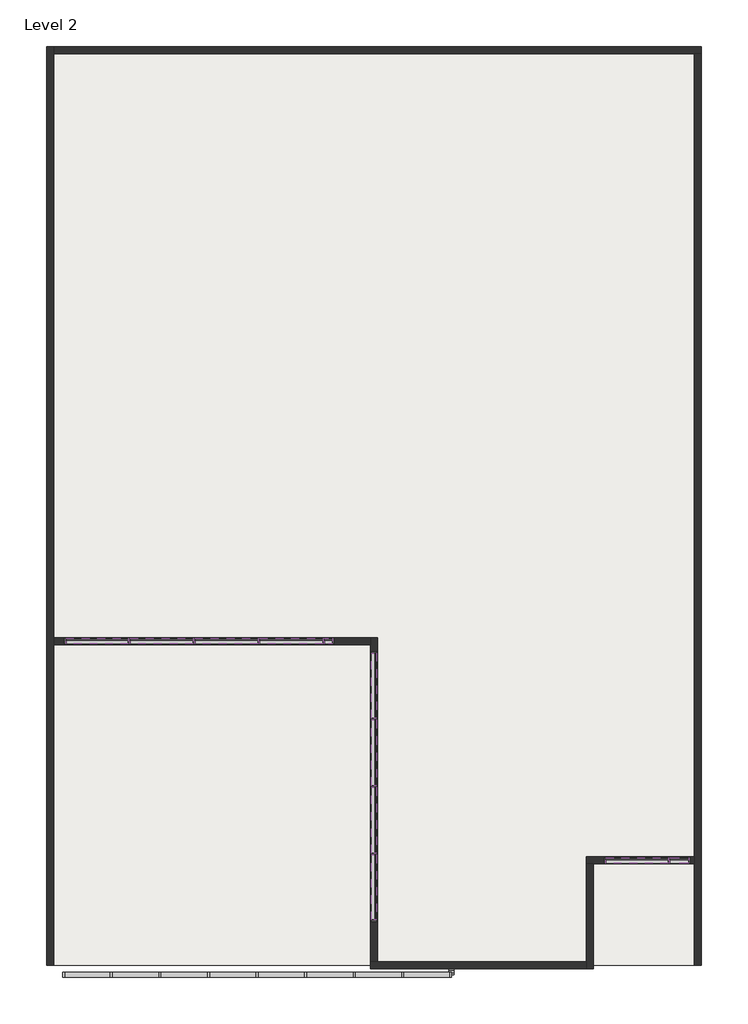
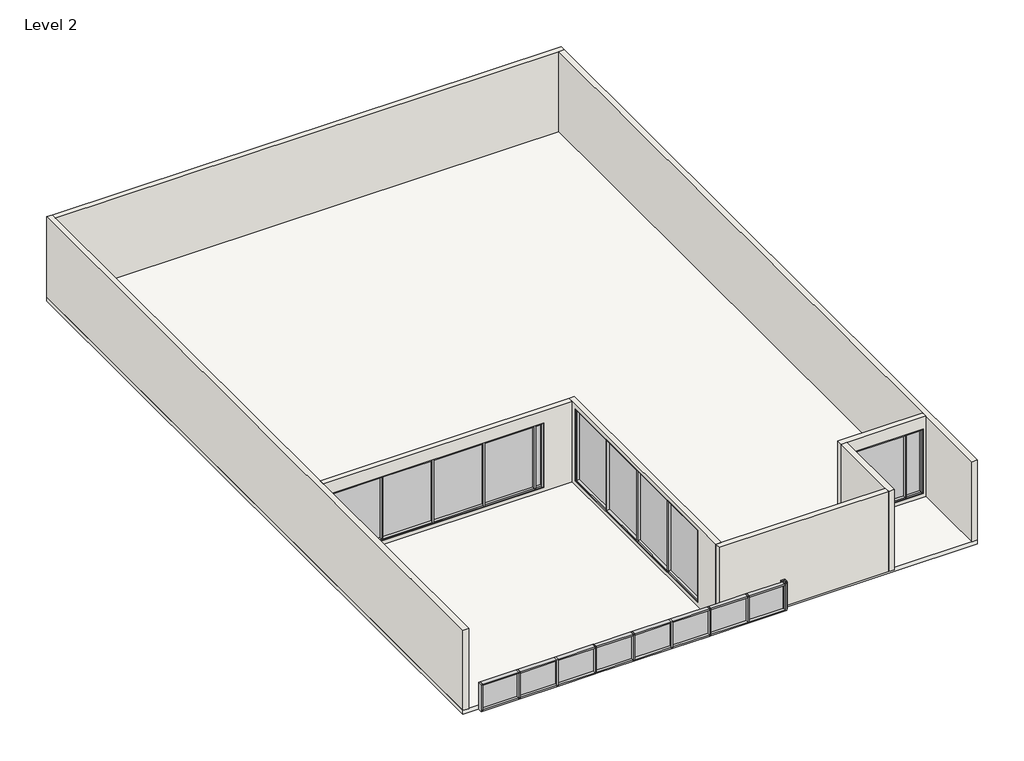
# One storey: 65 members, 20 plates, 8 walls, 1 slab.
"""IFC4 building model written with IfcOpenShell, lengths in millimetres."""

from ifc_helpers import new_model, si_unit, frame, origin, place, context, project, spatial, polyline, outline, extrude, faceted_brep, transform, mapped, element, save
from components import rectangular_mullion_50_x_150mm_ef1c4831, rectangular_mullion_50_x_150mm_86d49a4b, rectangular_mullion_50_x_150mm_a98d9a75, rectangular_mullion_50_x_150mm_ded00a16, rectangular_mullion_50_x_150mm_4a8db126, rectangular_mullion_50_x_150mm_15474f2d, rectangular_mullion_50_x_150mm_817551cd, rectangular_mullion_50_x_150mm_b402127a, rectangular_mullion_50_x_150mm_e4d4a7e6, rectangular_mullion_50_x_150mm_37458a5b, rectangular_mullion_50_x_150mm_e4b12c2e, rectangular_mullion_50_x_150mm_aaee7d48, rectangular_mullion_50_x_150mm_bcca0aad, rectangular_mullion_50_x_150mm_17218063, rectangular_mullion_50_x_150mm_0da89c4c, system_panel_glazed_91d575af, system_panel_glazed_99388aa9, system_panel_glazed_e22c965b, system_panel_glazed_90abe38c, system_panel_glazed_0f6e2381, system_panel_glazed_dc01897a, system_panel_glazed_f67349ae, system_panel_glazed_96f1d4d6, system_panel_glazed_c01e4bb7

model = new_model("IFC4")

# Units and contexts
model_context = context("Model", 3, world=origin())
ifc_project = project(units=[si_unit("LENGTHUNIT", "METRE", prefix="MILLI")], contexts=[model_context])

# Site, building, storey
site = spatial("IfcSite", under=ifc_project)
building = spatial("IfcBuilding", under=site)
storey = spatial("IfcBuildingStorey", under=building, Name="Level 2", Elevation=3048.0)

# Members
placement = place(None, origin())
rectangular_mullion_50_x_150mm_shape = rectangular_mullion_50_x_150mm_ef1c4831(model_context)
element("IfcMember", 1, ObjectType="Rectangular Mullion : 50 x 150mm", at=placement, inside=storey, context=model_context, shape_type="MappedRepresentation", body=[
    mapped(rectangular_mullion_50_x_150mm_shape, transform((-653.222521, -6711.5467593, 5638.8), x_axis=(0.0, 0.0, 1.0), y_axis=(0.0, -1.0, 0.0), z_axis=(1.0, 0.0, 0.0))),
])
rectangular_mullion_50_x_150mm_2_shape = rectangular_mullion_50_x_150mm_86d49a4b(model_context)
element("IfcMember", 2, ObjectType="Rectangular Mullion : 50 x 150mm", at=placement, inside=storey, context=model_context, shape_type="MappedRepresentation", body=[
    mapped(rectangular_mullion_50_x_150mm_2_shape, transform((-8173.222521, -6711.5467593, 3200.4), x_axis=(0.0, 0.0, -1.0), y_axis=(0.0, -1.0, 0.0), z_axis=(-1.0, 0.0, 0.0))),
])
element("IfcMember", 3, ObjectType="Rectangular Mullion : 50 x 150mm", at=placement, inside=storey, context=model_context, shape_type="MappedRepresentation", body=[
    mapped(rectangular_mullion_50_x_150mm_2_shape, transform((7066.777479, -12898.0177849, 3200.4), x_axis=(0.0, 0.0, -1.0), y_axis=(0.0, -1.0, 0.0), z_axis=(-1.0, 0.0, 0.0))),
])
rectangular_mullion_50_x_150mm_3_shape = rectangular_mullion_50_x_150mm_a98d9a75(model_context)
element("IfcMember", 4, ObjectType="Rectangular Mullion : 50 x 150mm", at=placement, inside=storey, context=model_context, shape_type="MappedRepresentation", body=[
    mapped(rectangular_mullion_50_x_150mm_3_shape, transform((-6393.222521, -6711.5467593, 3200.4), x_axis=(1.0, 0.0, 0.0), y_axis=(0.0, -1.0, 0.0), z_axis=(0.0, 0.0, -1.0))),
])
element("IfcMember", 5, ObjectType="Rectangular Mullion : 50 x 150mm", at=placement, inside=storey, context=model_context, shape_type="MappedRepresentation", body=[
    mapped(rectangular_mullion_50_x_150mm_3_shape, transform((-4563.222521, -6711.5467593, 3200.4), x_axis=(1.0, 0.0, 0.0), y_axis=(0.0, -1.0, 0.0), z_axis=(0.0, 0.0, -1.0))),
])
element("IfcMember", 6, ObjectType="Rectangular Mullion : 50 x 150mm", at=placement, inside=storey, context=model_context, shape_type="MappedRepresentation", body=[
    mapped(rectangular_mullion_50_x_150mm_3_shape, transform((-2733.222521, -6711.5467593, 3200.4), x_axis=(1.0, 0.0, 0.0), y_axis=(0.0, -1.0, 0.0), z_axis=(0.0, 0.0, -1.0))),
])
element("IfcMember", 7, ObjectType="Rectangular Mullion : 50 x 150mm", at=placement, inside=storey, context=model_context, shape_type="MappedRepresentation", body=[
    mapped(rectangular_mullion_50_x_150mm_3_shape, transform((-903.222521, -6711.5467593, 3200.4), x_axis=(1.0, 0.0, 0.0), y_axis=(0.0, -1.0, 0.0), z_axis=(0.0, 0.0, -1.0))),
])
element("IfcMember", 8, ObjectType="Rectangular Mullion : 50 x 150mm", at=placement, inside=storey, context=model_context, shape_type="MappedRepresentation", body=[
    mapped(rectangular_mullion_50_x_150mm_3_shape, transform((8846.777479, -12898.0177849, 3200.4), x_axis=(1.0, 0.0, 0.0), y_axis=(0.0, -1.0, 0.0), z_axis=(0.0, 0.0, -1.0))),
])
rectangular_mullion_50_x_150mm_4_shape = rectangular_mullion_50_x_150mm_ded00a16(model_context)
element("IfcMember", 9, ObjectType="Rectangular Mullion : 50 x 150mm", at=placement, inside=storey, context=model_context, shape_type="MappedRepresentation", body=[
    mapped(rectangular_mullion_50_x_150mm_4_shape, transform((-6368.222521, -6711.5467593, 3200.4), x_axis=(0.0, 0.0, -1.0), y_axis=(0.0, -1.0, 0.0), z_axis=(-1.0, 0.0, 0.0))),
])
element("IfcMember", 10, ObjectType="Rectangular Mullion : 50 x 150mm", at=placement, inside=storey, context=model_context, shape_type="MappedRepresentation", body=[
    mapped(rectangular_mullion_50_x_150mm_4_shape, transform((-4538.222521, -6711.5467593, 3200.4), x_axis=(0.0, 0.0, -1.0), y_axis=(0.0, -1.0, 0.0), z_axis=(-1.0, 0.0, 0.0))),
])
element("IfcMember", 11, ObjectType="Rectangular Mullion : 50 x 150mm", at=placement, inside=storey, context=model_context, shape_type="MappedRepresentation", body=[
    mapped(rectangular_mullion_50_x_150mm_4_shape, transform((-2708.222521, -6711.5467593, 3200.4), x_axis=(0.0, 0.0, -1.0), y_axis=(0.0, -1.0, 0.0), z_axis=(-1.0, 0.0, 0.0))),
])
element("IfcMember", 12, ObjectType="Rectangular Mullion : 50 x 150mm", at=placement, inside=storey, context=model_context, shape_type="MappedRepresentation", body=[
    mapped(rectangular_mullion_50_x_150mm_shape, transform((-878.222521, -6711.5467593, 3200.4), x_axis=(0.0, 0.0, -1.0), y_axis=(0.0, -1.0, 0.0), z_axis=(-1.0, 0.0, 0.0))),
])
element("IfcMember", 13, ObjectType="Rectangular Mullion : 50 x 150mm", at=placement, inside=storey, context=model_context, shape_type="MappedRepresentation", body=[
    mapped(rectangular_mullion_50_x_150mm_2_shape, transform((-6418.222521, -6711.5467593, 5638.8), x_axis=(0.0, 0.0, 1.0), y_axis=(0.0, -1.0, 0.0), z_axis=(1.0, 0.0, 0.0))),
])
element("IfcMember", 14, ObjectType="Rectangular Mullion : 50 x 150mm", at=placement, inside=storey, context=model_context, shape_type="MappedRepresentation", body=[
    mapped(rectangular_mullion_50_x_150mm_2_shape, transform((8821.777479, -12898.0177849, 5638.8), x_axis=(0.0, 0.0, 1.0), y_axis=(0.0, -1.0, 0.0), z_axis=(1.0, 0.0, 0.0))),
])
element("IfcMember", 15, ObjectType="Rectangular Mullion : 50 x 150mm", at=placement, inside=storey, context=model_context, shape_type="MappedRepresentation", body=[
    mapped(rectangular_mullion_50_x_150mm_4_shape, transform((-4588.222521, -6711.5467593, 5638.8), x_axis=(0.0, 0.0, 1.0), y_axis=(0.0, -1.0, 0.0), z_axis=(1.0, 0.0, 0.0))),
])
element("IfcMember", 16, ObjectType="Rectangular Mullion : 50 x 150mm", at=placement, inside=storey, context=model_context, shape_type="MappedRepresentation", body=[
    mapped(rectangular_mullion_50_x_150mm_4_shape, transform((-2758.222521, -6711.5467593, 5638.8), x_axis=(0.0, 0.0, 1.0), y_axis=(0.0, -1.0, 0.0), z_axis=(1.0, 0.0, 0.0))),
])
element("IfcMember", 17, ObjectType="Rectangular Mullion : 50 x 150mm", at=placement, inside=storey, context=model_context, shape_type="MappedRepresentation", body=[
    mapped(rectangular_mullion_50_x_150mm_4_shape, transform((-928.222521, -6711.5467593, 5638.8), x_axis=(0.0, 0.0, 1.0), y_axis=(0.0, -1.0, 0.0), z_axis=(1.0, 0.0, 0.0))),
])
rectangular_mullion_50_x_150mm_5_shape = rectangular_mullion_50_x_150mm_4a8db126(model_context)
element("IfcMember", 18, ObjectType="Rectangular Mullion : 50 x 150mm", at=placement, inside=storey, context=model_context, shape_type="MappedRepresentation", body=[
    mapped(rectangular_mullion_50_x_150mm_5_shape, transform((-8223.222521, -6711.5467593, 5638.8), x_axis=(-1.0, 0.0, 0.0), y_axis=(0.0, -1.0, 0.0), z_axis=(0.0, 0.0, 1.0))),
])
element("IfcMember", 19, ObjectType="Rectangular Mullion : 50 x 150mm", at=placement, inside=storey, context=model_context, shape_type="MappedRepresentation", body=[
    mapped(rectangular_mullion_50_x_150mm_5_shape, transform((7016.777479, -12898.0177849, 5638.8), x_axis=(-1.0, 0.0, 0.0), y_axis=(0.0, -1.0, 0.0), z_axis=(0.0, 0.0, 1.0))),
])
element("IfcMember", 20, ObjectType="Rectangular Mullion : 50 x 150mm", at=placement, inside=storey, context=model_context, shape_type="MappedRepresentation", body=[
    mapped(rectangular_mullion_50_x_150mm_5_shape, transform((-603.222521, -6711.5467593, 3200.4), x_axis=(1.0, 0.0, 0.0), y_axis=(0.0, -1.0, 0.0), z_axis=(0.0, 0.0, -1.0))),
])
element("IfcMember", 21, ObjectType="Rectangular Mullion : 50 x 150mm", at=placement, inside=storey, context=model_context, shape_type="MappedRepresentation", body=[
    mapped(rectangular_mullion_50_x_150mm_5_shape, transform((9455.177479, -12898.0177849, 3200.4), x_axis=(1.0, 0.0, 0.0), y_axis=(0.0, -1.0, 0.0), z_axis=(0.0, 0.0, -1.0))),
])
rectangular_mullion_50_x_150mm_6_shape = rectangular_mullion_50_x_150mm_15474f2d(model_context)
element("IfcMember", 22, ObjectType="Rectangular Mullion : 50 x 150mm", at=placement, inside=storey, context=model_context, shape_type="MappedRepresentation", body=[
    mapped(rectangular_mullion_50_x_150mm_6_shape, transform((9405.177479, -12898.0177849, 5638.8), x_axis=(0.0, 0.0, 1.0), y_axis=(0.0, -1.0, 0.0), z_axis=(1.0, 0.0, 0.0))),
])
element("IfcMember", 23, ObjectType="Rectangular Mullion : 50 x 150mm", at=placement, inside=storey, context=model_context, shape_type="MappedRepresentation", body=[
    mapped(rectangular_mullion_50_x_150mm_6_shape, transform((8871.777479, -12898.0177849, 3200.4), x_axis=(0.0, 0.0, -1.0), y_axis=(0.0, -1.0, 0.0), z_axis=(-1.0, 0.0, 0.0))),
])
rectangular_mullion_50_x_150mm_7_shape = rectangular_mullion_50_x_150mm_817551cd(model_context)
element("IfcMember", 24, ObjectType="Rectangular Mullion : 50 x 150mm", at=placement, inside=storey, context=model_context, shape_type="MappedRepresentation", body=[
    mapped(rectangular_mullion_50_x_150mm_7_shape, transform((2651.977479, -16123.9620478, 4075.5595785), x_axis=(0.0, 0.0, 1.0), y_axis=(0.0, -1.0, 0.0), z_axis=(1.0, 0.0, 0.0))),
])
element("IfcMember", 25, ObjectType="Rectangular Mullion : 50 x 150mm", at=placement, inside=storey, context=model_context, shape_type="MappedRepresentation", body=[
    mapped(rectangular_mullion_50_x_150mm_7_shape, transform((-6924.222521, -16123.9620478, 4075.5595785), x_axis=(0.0, 0.0, 1.0), y_axis=(0.0, -1.0, 0.0), z_axis=(1.0, 0.0, 0.0))),
])
element("IfcMember", 26, ObjectType="Rectangular Mullion : 50 x 150mm", at=placement, inside=storey, context=model_context, shape_type="MappedRepresentation", body=[
    mapped(rectangular_mullion_50_x_150mm_7_shape, transform((-8220.822521, -16123.9620478, 3048.0), x_axis=(0.0, 0.0, -1.0), y_axis=(0.0, -1.0, 0.0), z_axis=(-1.0, 0.0, 0.0))),
])
element("IfcMember", 27, ObjectType="Rectangular Mullion : 50 x 150mm", at=placement, inside=storey, context=model_context, shape_type="MappedRepresentation", body=[
    mapped(rectangular_mullion_50_x_150mm_7_shape, transform((1355.377479, -16123.9620478, 3048.0), x_axis=(0.0, 0.0, -1.0), y_axis=(0.0, -1.0, 0.0), z_axis=(-1.0, 0.0, 0.0))),
])
rectangular_mullion_50_x_150mm_8_shape = rectangular_mullion_50_x_150mm_b402127a(model_context)
element("IfcMember", 28, ObjectType="Rectangular Mullion : 50 x 150mm", at=placement, inside=storey, context=model_context, shape_type="MappedRepresentation", body=[
    mapped(rectangular_mullion_50_x_150mm_8_shape, transform((-2784.422521, -16123.9620478, 3048.0), x_axis=(1.0, 0.0, 0.0), y_axis=(0.0, -1.0, 0.0), z_axis=(0.0, 0.0, -1.0))),
])
element("IfcMember", 29, ObjectType="Rectangular Mullion : 50 x 150mm", at=placement, inside=storey, context=model_context, shape_type="MappedRepresentation", body=[
    mapped(rectangular_mullion_50_x_150mm_8_shape, transform((-5527.622521, -16123.9620478, 3048.0), x_axis=(1.0, 0.0, 0.0), y_axis=(0.0, -1.0, 0.0), z_axis=(0.0, 0.0, -1.0))),
])
element("IfcMember", 30, ObjectType="Rectangular Mullion : 50 x 150mm", at=placement, inside=storey, context=model_context, shape_type="MappedRepresentation", body=[
    mapped(rectangular_mullion_50_x_150mm_8_shape, transform((-4156.022521, -16123.9620478, 3048.0), x_axis=(1.0, 0.0, 0.0), y_axis=(0.0, -1.0, 0.0), z_axis=(0.0, 0.0, -1.0))),
])
element("IfcMember", 31, ObjectType="Rectangular Mullion : 50 x 150mm", at=placement, inside=storey, context=model_context, shape_type="MappedRepresentation", body=[
    mapped(rectangular_mullion_50_x_150mm_8_shape, transform((-6899.222521, -16123.9620478, 3048.0), x_axis=(1.0, 0.0, 0.0), y_axis=(0.0, -1.0, 0.0), z_axis=(0.0, 0.0, -1.0))),
])
element("IfcMember", 32, ObjectType="Rectangular Mullion : 50 x 150mm", at=placement, inside=storey, context=model_context, shape_type="MappedRepresentation", body=[
    mapped(rectangular_mullion_50_x_150mm_8_shape, transform((-1412.822521, -16123.9620478, 3048.0), x_axis=(1.0, 0.0, 0.0), y_axis=(0.0, -1.0, 0.0), z_axis=(0.0, 0.0, -1.0))),
])
element("IfcMember", 33, ObjectType="Rectangular Mullion : 50 x 150mm", at=placement, inside=storey, context=model_context, shape_type="MappedRepresentation", body=[
    mapped(rectangular_mullion_50_x_150mm_8_shape, transform((-41.222521, -16123.9620478, 3048.0), x_axis=(1.0, 0.0, 0.0), y_axis=(0.0, -1.0, 0.0), z_axis=(0.0, 0.0, -1.0))),
])
element("IfcMember", 34, ObjectType="Rectangular Mullion : 50 x 150mm", at=placement, inside=storey, context=model_context, shape_type="MappedRepresentation", body=[
    mapped(rectangular_mullion_50_x_150mm_8_shape, transform((1330.377479, -16123.9620478, 3048.0), x_axis=(1.0, 0.0, 0.0), y_axis=(0.0, -1.0, 0.0), z_axis=(0.0, 0.0, -1.0))),
])
rectangular_mullion_50_x_150mm_9_shape = rectangular_mullion_50_x_150mm_e4d4a7e6(model_context)
element("IfcMember", 35, ObjectType="Rectangular Mullion : 50 x 150mm", at=placement, inside=storey, context=model_context, shape_type="MappedRepresentation", body=[
    mapped(rectangular_mullion_50_x_150mm_9_shape, transform((-2759.422521, -16123.9620478, 3048.0), x_axis=(0.0, 0.0, -1.0), y_axis=(0.0, -1.0, 0.0), z_axis=(-1.0, 0.0, 0.0))),
])
element("IfcMember", 36, ObjectType="Rectangular Mullion : 50 x 150mm", at=placement, inside=storey, context=model_context, shape_type="MappedRepresentation", body=[
    mapped(rectangular_mullion_50_x_150mm_9_shape, transform((-5502.622521, -16123.9620478, 3048.0), x_axis=(0.0, 0.0, -1.0), y_axis=(0.0, -1.0, 0.0), z_axis=(-1.0, 0.0, 0.0))),
])
element("IfcMember", 37, ObjectType="Rectangular Mullion : 50 x 150mm", at=placement, inside=storey, context=model_context, shape_type="MappedRepresentation", body=[
    mapped(rectangular_mullion_50_x_150mm_9_shape, transform((-4131.022521, -16123.9620478, 3048.0), x_axis=(0.0, 0.0, -1.0), y_axis=(0.0, -1.0, 0.0), z_axis=(-1.0, 0.0, 0.0))),
])
element("IfcMember", 38, ObjectType="Rectangular Mullion : 50 x 150mm", at=placement, inside=storey, context=model_context, shape_type="MappedRepresentation", body=[
    mapped(rectangular_mullion_50_x_150mm_9_shape, transform((-6874.222521, -16123.9620478, 3048.0), x_axis=(0.0, 0.0, -1.0), y_axis=(0.0, -1.0, 0.0), z_axis=(-1.0, 0.0, 0.0))),
])
element("IfcMember", 39, ObjectType="Rectangular Mullion : 50 x 150mm", at=placement, inside=storey, context=model_context, shape_type="MappedRepresentation", body=[
    mapped(rectangular_mullion_50_x_150mm_9_shape, transform((-1387.822521, -16123.9620478, 3048.0), x_axis=(0.0, 0.0, -1.0), y_axis=(0.0, -1.0, 0.0), z_axis=(-1.0, 0.0, 0.0))),
])
element("IfcMember", 40, ObjectType="Rectangular Mullion : 50 x 150mm", at=placement, inside=storey, context=model_context, shape_type="MappedRepresentation", body=[
    mapped(rectangular_mullion_50_x_150mm_9_shape, transform((-16.222521, -16123.9620478, 3048.0), x_axis=(0.0, 0.0, -1.0), y_axis=(0.0, -1.0, 0.0), z_axis=(-1.0, 0.0, 0.0))),
])
element("IfcMember", 41, ObjectType="Rectangular Mullion : 50 x 150mm", at=placement, inside=storey, context=model_context, shape_type="MappedRepresentation", body=[
    mapped(rectangular_mullion_50_x_150mm_9_shape, transform((-2809.422521, -16123.9620478, 4075.5595785), x_axis=(0.0, 0.0, 1.0), y_axis=(0.0, -1.0, 0.0), z_axis=(1.0, 0.0, 0.0))),
])
element("IfcMember", 42, ObjectType="Rectangular Mullion : 50 x 150mm", at=placement, inside=storey, context=model_context, shape_type="MappedRepresentation", body=[
    mapped(rectangular_mullion_50_x_150mm_9_shape, transform((-5552.622521, -16123.9620478, 4075.5595785), x_axis=(0.0, 0.0, 1.0), y_axis=(0.0, -1.0, 0.0), z_axis=(1.0, 0.0, 0.0))),
])
element("IfcMember", 43, ObjectType="Rectangular Mullion : 50 x 150mm", at=placement, inside=storey, context=model_context, shape_type="MappedRepresentation", body=[
    mapped(rectangular_mullion_50_x_150mm_9_shape, transform((-4181.022521, -16123.9620478, 4075.5595785), x_axis=(0.0, 0.0, 1.0), y_axis=(0.0, -1.0, 0.0), z_axis=(1.0, 0.0, 0.0))),
])
element("IfcMember", 44, ObjectType="Rectangular Mullion : 50 x 150mm", at=placement, inside=storey, context=model_context, shape_type="MappedRepresentation", body=[
    mapped(rectangular_mullion_50_x_150mm_9_shape, transform((-1437.822521, -16123.9620478, 4075.5595785), x_axis=(0.0, 0.0, 1.0), y_axis=(0.0, -1.0, 0.0), z_axis=(1.0, 0.0, 0.0))),
])
element("IfcMember", 45, ObjectType="Rectangular Mullion : 50 x 150mm", at=placement, inside=storey, context=model_context, shape_type="MappedRepresentation", body=[
    mapped(rectangular_mullion_50_x_150mm_9_shape, transform((-66.222521, -16123.9620478, 4075.5595785), x_axis=(0.0, 0.0, 1.0), y_axis=(0.0, -1.0, 0.0), z_axis=(1.0, 0.0, 0.0))),
])
element("IfcMember", 46, ObjectType="Rectangular Mullion : 50 x 150mm", at=placement, inside=storey, context=model_context, shape_type="MappedRepresentation", body=[
    mapped(rectangular_mullion_50_x_150mm_9_shape, transform((1305.377479, -16123.9620478, 4075.5595785), x_axis=(0.0, 0.0, 1.0), y_axis=(0.0, -1.0, 0.0), z_axis=(1.0, 0.0, 0.0))),
])
rectangular_mullion_50_x_150mm_10_shape = rectangular_mullion_50_x_150mm_37458a5b(model_context)
element("IfcMember", 47, ObjectType="Rectangular Mullion : 50 x 150mm", at=placement, inside=storey, context=model_context, shape_type="MappedRepresentation", body=[
    mapped(rectangular_mullion_50_x_150mm_10_shape, transform((-8270.822521, -16123.9620478, 4075.5595785), x_axis=(-1.0, 0.0, 0.0), y_axis=(0.0, -1.0, 0.0), z_axis=(0.0, 0.0, 1.0))),
])
element("IfcMember", 48, ObjectType="Rectangular Mullion : 50 x 150mm", at=placement, inside=storey, context=model_context, shape_type="MappedRepresentation", body=[
    mapped(rectangular_mullion_50_x_150mm_10_shape, transform((2701.977479, -16123.9620478, 4075.5595785), x_axis=(0.0, -1.0, 0.0), y_axis=(1.0, 0.0, 0.0), z_axis=(0.0, 0.0, 1.0))),
])
element("IfcMember", 49, ObjectType="Rectangular Mullion : 50 x 150mm", at=placement, inside=storey, context=model_context, shape_type="MappedRepresentation", body=[
    mapped(rectangular_mullion_50_x_150mm_10_shape, transform((2701.977479, -16123.9620478, 3048.0), x_axis=(1.0, 0.0, 0.0), y_axis=(0.0, -1.0, 0.0), z_axis=(0.0, 0.0, -1.0))),
])
element("IfcMember", 50, ObjectType="Rectangular Mullion : 50 x 150mm", at=placement, inside=storey, context=model_context, shape_type="MappedRepresentation", body=[
    mapped(rectangular_mullion_50_x_150mm_10_shape, transform((2701.977479, -15955.5467593, 3048.0), x_axis=(0.0, 1.0, 0.0), y_axis=(1.0, 0.0, 0.0), z_axis=(0.0, 0.0, -1.0))),
])
rectangular_mullion_50_x_150mm_11_shape = rectangular_mullion_50_x_150mm_e4b12c2e(model_context)
element("IfcMember", 51, ObjectType="Rectangular Mullion : 50 x 150mm", at=placement, inside=storey, context=model_context, shape_type="MappedRepresentation", body=[
    mapped(rectangular_mullion_50_x_150mm_11_shape, transform((2701.977479, -16005.5467593, 4075.5595785), x_axis=(0.0, 0.0, 1.0), y_axis=(1.0, 0.0, 0.0), z_axis=(0.0, 1.0, 0.0))),
])
element("IfcMember", 52, ObjectType="Rectangular Mullion : 50 x 150mm", at=placement, inside=storey, context=model_context, shape_type="MappedRepresentation", body=[
    mapped(rectangular_mullion_50_x_150mm_11_shape, transform((2701.977479, -16073.9620478, 3048.0), x_axis=(0.0, 0.0, -1.0), y_axis=(1.0, 0.0, 0.0), z_axis=(0.0, -1.0, 0.0))),
])
rectangular_mullion_50_x_150mm_12_shape = rectangular_mullion_50_x_150mm_aaee7d48(model_context)
element("IfcMember", 53, ObjectType="Rectangular Mullion : 50 x 150mm", at=placement, inside=storey, context=model_context, shape_type="MappedRepresentation", body=[
    mapped(rectangular_mullion_50_x_150mm_12_shape, transform((515.977479, -14573.2177849, 5943.6), x_axis=(0.0, 0.0, 1.0), y_axis=(-1.0, 0.0, 0.0), z_axis=(0.0, -1.0, 0.0))),
])
element("IfcMember", 54, ObjectType="Rectangular Mullion : 50 x 150mm", at=placement, inside=storey, context=model_context, shape_type="MappedRepresentation", body=[
    mapped(rectangular_mullion_50_x_150mm_12_shape, transform((515.977479, -8883.2177849, 5943.6), x_axis=(0.0, 0.0, 1.0), y_axis=(-1.0, 0.0, 0.0), z_axis=(0.0, -1.0, 0.0))),
])
element("IfcMember", 55, ObjectType="Rectangular Mullion : 50 x 150mm", at=placement, inside=storey, context=model_context, shape_type="MappedRepresentation", body=[
    mapped(rectangular_mullion_50_x_150mm_12_shape, transform((515.977479, -7053.2177849, 3200.4), x_axis=(0.0, 0.0, -1.0), y_axis=(-1.0, 0.0, 0.0), z_axis=(0.0, 1.0, 0.0))),
])
element("IfcMember", 56, ObjectType="Rectangular Mullion : 50 x 150mm", at=placement, inside=storey, context=model_context, shape_type="MappedRepresentation", body=[
    mapped(rectangular_mullion_50_x_150mm_12_shape, transform((515.977479, -12743.2177849, 3200.4), x_axis=(0.0, 0.0, -1.0), y_axis=(-1.0, 0.0, 0.0), z_axis=(0.0, 1.0, 0.0))),
])
rectangular_mullion_50_x_150mm_13_shape = rectangular_mullion_50_x_150mm_bcca0aad(model_context)
element("IfcMember", 57, ObjectType="Rectangular Mullion : 50 x 150mm", at=placement, inside=storey, context=model_context, shape_type="MappedRepresentation", body=[
    mapped(rectangular_mullion_50_x_150mm_13_shape, transform((515.977479, -10813.2177849, 3200.4), x_axis=(0.0, -1.0, 0.0), y_axis=(-1.0, 0.0, 0.0), z_axis=(0.0, 0.0, -1.0))),
])
element("IfcMember", 58, ObjectType="Rectangular Mullion : 50 x 150mm", at=placement, inside=storey, context=model_context, shape_type="MappedRepresentation", body=[
    mapped(rectangular_mullion_50_x_150mm_13_shape, transform((515.977479, -8908.2177849, 3200.4), x_axis=(0.0, -1.0, 0.0), y_axis=(-1.0, 0.0, 0.0), z_axis=(0.0, 0.0, -1.0))),
])
element("IfcMember", 59, ObjectType="Rectangular Mullion : 50 x 150mm", at=placement, inside=storey, context=model_context, shape_type="MappedRepresentation", body=[
    mapped(rectangular_mullion_50_x_150mm_13_shape, transform((515.977479, -12718.2177849, 3200.4), x_axis=(0.0, -1.0, 0.0), y_axis=(-1.0, 0.0, 0.0), z_axis=(0.0, 0.0, -1.0))),
])
rectangular_mullion_50_x_150mm_14_shape = rectangular_mullion_50_x_150mm_17218063(model_context)
element("IfcMember", 60, ObjectType="Rectangular Mullion : 50 x 150mm", at=placement, inside=storey, context=model_context, shape_type="MappedRepresentation", body=[
    mapped(rectangular_mullion_50_x_150mm_14_shape, transform((515.977479, -10838.2177849, 3200.4), x_axis=(0.0, 0.0, -1.0), y_axis=(-1.0, 0.0, 0.0), z_axis=(0.0, 1.0, 0.0))),
])
element("IfcMember", 61, ObjectType="Rectangular Mullion : 50 x 150mm", at=placement, inside=storey, context=model_context, shape_type="MappedRepresentation", body=[
    mapped(rectangular_mullion_50_x_150mm_14_shape, transform((515.977479, -8933.2177849, 3200.4), x_axis=(0.0, 0.0, -1.0), y_axis=(-1.0, 0.0, 0.0), z_axis=(0.0, 1.0, 0.0))),
])
element("IfcMember", 62, ObjectType="Rectangular Mullion : 50 x 150mm", at=placement, inside=storey, context=model_context, shape_type="MappedRepresentation", body=[
    mapped(rectangular_mullion_50_x_150mm_14_shape, transform((515.977479, -10788.2177849, 5943.6), x_axis=(0.0, 0.0, 1.0), y_axis=(-1.0, 0.0, 0.0), z_axis=(0.0, -1.0, 0.0))),
])
element("IfcMember", 63, ObjectType="Rectangular Mullion : 50 x 150mm", at=placement, inside=storey, context=model_context, shape_type="MappedRepresentation", body=[
    mapped(rectangular_mullion_50_x_150mm_14_shape, transform((515.977479, -12693.2177849, 5943.6), x_axis=(0.0, 0.0, 1.0), y_axis=(-1.0, 0.0, 0.0), z_axis=(0.0, -1.0, 0.0))),
])
rectangular_mullion_50_x_150mm_15_shape = rectangular_mullion_50_x_150mm_0da89c4c(model_context)
element("IfcMember", 64, ObjectType="Rectangular Mullion : 50 x 150mm", at=placement, inside=storey, context=model_context, shape_type="MappedRepresentation", body=[
    mapped(rectangular_mullion_50_x_150mm_15_shape, transform((515.977479, -7003.2177849, 5943.6), x_axis=(0.0, 1.0, 0.0), y_axis=(-1.0, 0.0, 0.0), z_axis=(0.0, 0.0, 1.0))),
])
element("IfcMember", 65, ObjectType="Rectangular Mullion : 50 x 150mm", at=placement, inside=storey, context=model_context, shape_type="MappedRepresentation", body=[
    mapped(rectangular_mullion_50_x_150mm_15_shape, transform((515.977479, -14623.2177849, 3200.4), x_axis=(0.0, -1.0, 0.0), y_axis=(-1.0, 0.0, 0.0), z_axis=(0.0, 0.0, -1.0))),
])

# Plates
system_panel_glazed_shape = system_panel_glazed_91d575af(model_context)
element("IfcPlate", 66, ObjectType="System Panel : Glazed", at=placement, inside=storey, context=model_context, shape_type="MappedRepresentation", body=[
    mapped(system_panel_glazed_shape, transform((-7295.722521, -6711.5467593, 3250.4), x_axis=(1.0, 0.0, 0.0), y_axis=(0.0, 1.0, 0.0), z_axis=(0.0, 0.0, 1.0))),
])
element("IfcPlate", 67, ObjectType="System Panel : Glazed", at=placement, inside=storey, context=model_context, shape_type="MappedRepresentation", body=[
    mapped(system_panel_glazed_shape, transform((7944.277479, -12898.0177849, 3250.4), x_axis=(1.0, 0.0, 0.0), y_axis=(0.0, 1.0, 0.0), z_axis=(0.0, 0.0, 1.0))),
])
system_panel_glazed_2_shape = system_panel_glazed_99388aa9(model_context)
element("IfcPlate", 68, ObjectType="System Panel : Glazed", at=placement, inside=storey, context=model_context, shape_type="MappedRepresentation", body=[
    mapped(system_panel_glazed_2_shape, transform((-5478.222521, -6711.5467593, 3250.4), x_axis=(1.0, 0.0, 0.0), y_axis=(0.0, 1.0, 0.0), z_axis=(0.0, 0.0, 1.0))),
])
element("IfcPlate", 69, ObjectType="System Panel : Glazed", at=placement, inside=storey, context=model_context, shape_type="MappedRepresentation", body=[
    mapped(system_panel_glazed_2_shape, transform((-3648.222521, -6711.5467593, 3250.4), x_axis=(1.0, 0.0, 0.0), y_axis=(0.0, 1.0, 0.0), z_axis=(0.0, 0.0, 1.0))),
])
element("IfcPlate", 70, ObjectType="System Panel : Glazed", at=placement, inside=storey, context=model_context, shape_type="MappedRepresentation", body=[
    mapped(system_panel_glazed_2_shape, transform((-1818.222521, -6711.5467593, 3250.4), x_axis=(1.0, 0.0, 0.0), y_axis=(0.0, 1.0, 0.0), z_axis=(0.0, 0.0, 1.0))),
])
system_panel_glazed_3_shape = system_panel_glazed_e22c965b(model_context)
element("IfcPlate", 71, ObjectType="System Panel : Glazed", at=placement, inside=storey, context=model_context, shape_type="MappedRepresentation", body=[
    mapped(system_panel_glazed_3_shape, transform((-765.722521, -6711.5467593, 3250.4), x_axis=(1.0, 0.0, 0.0), y_axis=(0.0, 1.0, 0.0), z_axis=(0.0, 0.0, 1.0))),
])
system_panel_glazed_4_shape = system_panel_glazed_90abe38c(model_context)
element("IfcPlate", 72, ObjectType="System Panel : Glazed", at=placement, inside=storey, context=model_context, shape_type="MappedRepresentation", body=[
    mapped(system_panel_glazed_4_shape, transform((9138.477479, -12898.0177849, 3250.4), x_axis=(1.0, 0.0, 0.0), y_axis=(0.0, 1.0, 0.0), z_axis=(0.0, 0.0, 1.0))),
])
system_panel_glazed_5_shape = system_panel_glazed_0f6e2381(model_context)
element("IfcPlate", 73, ObjectType="System Panel : Glazed", at=placement, inside=storey, context=model_context, shape_type="MappedRepresentation", body=[
    mapped(system_panel_glazed_5_shape, transform((-7572.522521, -16123.9620478, 3098.0), x_axis=(1.0, 0.0, 0.0), y_axis=(0.0, 1.0, 0.0), z_axis=(0.0, 0.0, 1.0))),
])
element("IfcPlate", 74, ObjectType="System Panel : Glazed", at=placement, inside=storey, context=model_context, shape_type="MappedRepresentation", body=[
    mapped(system_panel_glazed_5_shape, transform((2003.677479, -16123.9620478, 3098.0), x_axis=(1.0, 0.0, 0.0), y_axis=(0.0, 1.0, 0.0), z_axis=(0.0, 0.0, 1.0))),
])
system_panel_glazed_6_shape = system_panel_glazed_dc01897a(model_context)
element("IfcPlate", 75, ObjectType="System Panel : Glazed", at=placement, inside=storey, context=model_context, shape_type="MappedRepresentation", body=[
    mapped(system_panel_glazed_6_shape, transform((-2098.622521, -16123.9620478, 3098.0), x_axis=(1.0, 0.0, 0.0), y_axis=(0.0, 1.0, 0.0), z_axis=(0.0, 0.0, 1.0))),
])
element("IfcPlate", 76, ObjectType="System Panel : Glazed", at=placement, inside=storey, context=model_context, shape_type="MappedRepresentation", body=[
    mapped(system_panel_glazed_6_shape, transform((-4841.822521, -16123.9620478, 3098.0), x_axis=(1.0, 0.0, 0.0), y_axis=(0.0, 1.0, 0.0), z_axis=(0.0, 0.0, 1.0))),
])
element("IfcPlate", 77, ObjectType="System Panel : Glazed", at=placement, inside=storey, context=model_context, shape_type="MappedRepresentation", body=[
    mapped(system_panel_glazed_6_shape, transform((-3470.222521, -16123.9620478, 3098.0), x_axis=(1.0, 0.0, 0.0), y_axis=(0.0, 1.0, 0.0), z_axis=(0.0, 0.0, 1.0))),
])
element("IfcPlate", 78, ObjectType="System Panel : Glazed", at=placement, inside=storey, context=model_context, shape_type="MappedRepresentation", body=[
    mapped(system_panel_glazed_6_shape, transform((-6213.422521, -16123.9620478, 3098.0), x_axis=(1.0, 0.0, 0.0), y_axis=(0.0, 1.0, 0.0), z_axis=(0.0, 0.0, 1.0))),
])
element("IfcPlate", 79, ObjectType="System Panel : Glazed", at=placement, inside=storey, context=model_context, shape_type="MappedRepresentation", body=[
    mapped(system_panel_glazed_6_shape, transform((-727.022521, -16123.9620478, 3098.0), x_axis=(1.0, 0.0, 0.0), y_axis=(0.0, 1.0, 0.0), z_axis=(0.0, 0.0, 1.0))),
])
element("IfcPlate", 80, ObjectType="System Panel : Glazed", at=placement, inside=storey, context=model_context, shape_type="MappedRepresentation", body=[
    mapped(system_panel_glazed_6_shape, transform((644.577479, -16123.9620478, 3098.0), x_axis=(1.0, 0.0, 0.0), y_axis=(0.0, 1.0, 0.0), z_axis=(0.0, 0.0, 1.0))),
])
system_panel_glazed_7_shape = system_panel_glazed_f67349ae(model_context)
element("IfcPlate", 81, ObjectType="System Panel : Glazed", at=placement, inside=storey, context=model_context, shape_type="MappedRepresentation", body=[
    mapped(system_panel_glazed_7_shape, transform((2701.977479, -16039.7544035, 3098.0), x_axis=(0.0, 1.0, 0.0), y_axis=(-1.0, 0.0, 0.0), z_axis=(0.0, 0.0, 1.0))),
])
system_panel_glazed_8_shape = system_panel_glazed_96f1d4d6(model_context)
element("IfcPlate", 82, ObjectType="System Panel : Glazed", at=placement, inside=storey, context=model_context, shape_type="MappedRepresentation", body=[
    mapped(system_panel_glazed_8_shape, transform((515.977479, -7968.2177849, 3250.4), x_axis=(0.0, -1.0, 0.0), y_axis=(1.0, 0.0, 0.0), z_axis=(0.0, 0.0, 1.0))),
])
element("IfcPlate", 83, ObjectType="System Panel : Glazed", at=placement, inside=storey, context=model_context, shape_type="MappedRepresentation", body=[
    mapped(system_panel_glazed_8_shape, transform((515.977479, -13658.2177849, 3250.4), x_axis=(0.0, -1.0, 0.0), y_axis=(1.0, 0.0, 0.0), z_axis=(0.0, 0.0, 1.0))),
])
system_panel_glazed_9_shape = system_panel_glazed_c01e4bb7(model_context)
element("IfcPlate", 84, ObjectType="System Panel : Glazed", at=placement, inside=storey, context=model_context, shape_type="MappedRepresentation", body=[
    mapped(system_panel_glazed_9_shape, transform((515.977479, -11765.7177849, 3250.4), x_axis=(0.0, -1.0, 0.0), y_axis=(1.0, 0.0, 0.0), z_axis=(0.0, 0.0, 1.0))),
])
element("IfcPlate", 85, ObjectType="System Panel : Glazed", at=placement, inside=storey, context=model_context, shape_type="MappedRepresentation", body=[
    mapped(system_panel_glazed_9_shape, transform((515.977479, -9860.7177849, 3250.4), x_axis=(0.0, -1.0, 0.0), y_axis=(1.0, 0.0, 0.0), z_axis=(0.0, 0.0, 1.0))),
])

# Slab
element("IfcSlab", 86, ObjectType="Generic 150mm", at=placement, inside=storey, context=model_context, shape_type="SweptSolid", body=[
    extrude(outline(polyline([(-8728.022521, 10061.9822151), (9759.977479, 10061.9822151), (9759.977479, -15855.5467593), (-8728.022521, -15855.5467593), (-8728.022521, 10061.9822151)])), frame((0.0, 0.0, 2895.6), z_axis=(0.0, 0.0, 1.0), x_axis=(1.0, 0.0, 0.0)), (0.0, 0.0, 1.0), 152.4),
])

# Walls
element("IfcWall", 87, ObjectType="Generic - 200mm", at=placement, inside=storey, context=model_context, shape_type="Brep", body=[
    faceted_brep([(-8728.022521, 10061.9822151, 3048.0), (-8728.022521, -15855.5467593, 3048.0), (-8728.022521, -15855.5467593, 6096.0), (-8728.022521, 10061.9822151, 6096.0), (-8528.022521, 10061.9822151, 3048.0), (-8528.022521, 10061.9822151, 6096.0), (-8528.022521, 9861.9822151, 6096.0), (-8528.022521, -6611.5467593, 6096.0), (-8528.022521, -6811.5467593, 6096.0), (-8528.022521, -15855.5467593, 6096.0), (-8528.022521, -15855.5467593, 3048.0), (-8528.022521, -6811.5467593, 3048.0), (-8528.022521, -6611.5467593, 3048.0), (-8528.022521, 9861.9822151, 3048.0)], [[[0, 1, 2, 3]], [[4, 5, 6, 7, 8, 9, 10, 11, 12, 13]], [[1, 0, 4, 13, 12, 11, 10]], [[2, 1, 10, 9]], [[3, 2, 9, 8, 7, 6, 5]], [[0, 3, 5, 4]]]),
])
element("IfcWall", 88, ObjectType="Generic - 200mm", at=placement, inside=storey, context=model_context, shape_type="Brep", body=[
    faceted_brep([(-8528.022521, 9861.9822151, 3048.0), (9559.977479, 9861.9822151, 3048.0), (9759.977479, 9861.9822151, 3048.0), (9759.977479, 9861.9822151, 6096.0), (9559.977479, 9861.9822151, 6096.0), (-8528.022521, 9861.9822151, 6096.0), (-8528.022521, 10061.9822151, 3048.0), (-8528.022521, 10061.9822151, 6096.0), (9759.977479, 10061.9822151, 6096.0), (9759.977479, 10061.9822151, 3048.0)], [[[0, 1, 2, 3, 4, 5]], [[6, 7, 8, 9]], [[2, 1, 0, 6, 9]], [[5, 4, 3, 8, 7]], [[0, 5, 7, 6]], [[3, 2, 9, 8]]]),
])
element("IfcWall", 89, ObjectType="Generic - 200mm", at=placement, inside=storey, context=model_context, shape_type="Brep", body=[
    faceted_brep([(9559.977479, 9861.9822151, 3048.0), (9559.977479, -12798.0177849, 3048.0), (9559.977479, -12998.0177849, 3048.0), (9559.977479, -15855.5467593, 3048.0), (9559.977479, -15855.5467593, 6096.0), (9559.977479, -12998.0177849, 6096.0), (9559.977479, -12798.0177849, 6096.0), (9559.977479, 9861.9822151, 6096.0), (9759.977479, 9861.9822151, 3048.0), (9759.977479, 9861.9822151, 6096.0), (9759.977479, -15855.5467593, 6096.0), (9759.977479, -15855.5467593, 3048.0)], [[[0, 1, 2, 3, 4, 5, 6, 7]], [[8, 9, 10, 11]], [[3, 2, 1, 0, 8, 11]], [[4, 3, 11, 10]], [[7, 6, 5, 4, 10, 9]], [[0, 7, 9, 8]]]),
])
element("IfcWall", 90, ObjectType="Generic - 200mm", at=placement, inside=storey, context=model_context, shape_type="Brep", body=[
    faceted_brep([(9559.977479, -12798.0177849, 3048.0), (6511.977479, -12798.0177849, 3048.0), (6511.977479, -12798.0177849, 6096.0), (9559.977479, -12798.0177849, 6096.0), (7016.777479, -12798.0177849, 5638.8), (7016.777479, -12798.0177849, 3200.4), (9455.177479, -12798.0177849, 3200.4), (9455.177479, -12798.0177849, 5638.8), (6511.977479, -12998.0177849, 3048.0), (6711.977479, -12998.0177849, 3048.0), (9559.977479, -12998.0177849, 3048.0), (9559.977479, -12998.0177849, 6096.0), (6711.977479, -12998.0177849, 6096.0), (6511.977479, -12998.0177849, 6096.0), (7016.777479, -12998.0177849, 3200.4), (7016.777479, -12998.0177849, 5638.8), (9455.177479, -12998.0177849, 5638.8), (9455.177479, -12998.0177849, 3200.4)], [[[0, 1, 2, 3], [4, 5, 6, 7]], [[8, 9, 10, 11, 12, 13], [14, 15, 16, 17]], [[1, 0, 10, 9, 8]], [[3, 2, 13, 12, 11]], [[0, 3, 11, 10]], [[2, 1, 8, 13]], [[14, 5, 4, 15]], [[15, 4, 7, 16]], [[16, 7, 6, 17]], [[5, 14, 17, 6]]]),
])
element("IfcWall", 91, ObjectType="Generic - 200mm", at=placement, inside=storey, context=model_context, shape_type="Brep", body=[
    faceted_brep([(6511.977479, -12998.0177849, 3048.0), (6511.977479, -15755.5467593, 3048.0), (6511.977479, -15955.5467593, 3048.0), (6511.977479, -15955.5467593, 6096.0), (6511.977479, -15755.5467593, 6096.0), (6511.977479, -12998.0177849, 6096.0), (6711.977479, -12998.0177849, 3048.0), (6711.977479, -12998.0177849, 6096.0), (6711.977479, -15955.5467593, 6096.0), (6711.977479, -15955.5467593, 3048.0)], [[[0, 1, 2, 3, 4, 5]], [[6, 7, 8, 9]], [[2, 1, 0, 6, 9]], [[5, 4, 3, 8, 7]], [[0, 5, 7, 6]], [[3, 2, 9, 8]]]),
])
element("IfcWall", 92, ObjectType="Generic - 200mm", at=placement, inside=storey, context=model_context, shape_type="Brep", body=[
    faceted_brep([(6511.977479, -15755.5467593, 3048.0), (615.977479, -15755.5467593, 3048.0), (415.977479, -15755.5467593, 3048.0), (415.977479, -15755.5467593, 6096.0), (615.977479, -15755.5467593, 6096.0), (6511.977479, -15755.5467593, 6096.0), (6511.977479, -15955.5467593, 3048.0), (6511.977479, -15955.5467593, 6096.0), (415.977479, -15955.5467593, 6096.0), (415.977479, -15955.5467593, 3048.0)], [[[0, 1, 2, 3, 4, 5]], [[6, 7, 8, 9]], [[2, 1, 0, 6, 9]], [[5, 4, 3, 8, 7]], [[0, 5, 7, 6]], [[3, 2, 9, 8]]]),
])
element("IfcWall", 93, ObjectType="Generic - 200mm", at=placement, inside=storey, context=model_context, shape_type="Brep", body=[
    faceted_brep([(615.977479, -15755.5467593, 3048.0), (615.977479, -6611.5467593, 3048.0), (615.977479, -6611.5467593, 6096.0), (615.977479, -15755.5467593, 6096.0), (615.977479, -7003.2177849, 5943.6), (615.977479, -7003.2177849, 3200.4), (615.977479, -14623.2177849, 3200.4), (615.977479, -14623.2177849, 5943.6), (415.977479, -6611.5467593, 3048.0), (415.977479, -6811.5467593, 3048.0), (415.977479, -15755.5467593, 3048.0), (415.977479, -15755.5467593, 6096.0), (415.977479, -6811.5467593, 6096.0), (415.977479, -6611.5467593, 6096.0), (415.977479, -7003.2177849, 3200.4), (415.977479, -7003.2177849, 5943.6), (415.977479, -14623.2177849, 5943.6), (415.977479, -14623.2177849, 3200.4)], [[[0, 1, 2, 3], [4, 5, 6, 7]], [[8, 9, 10, 11, 12, 13], [14, 15, 16, 17]], [[1, 0, 10, 9, 8]], [[3, 2, 13, 12, 11]], [[0, 3, 11, 10]], [[2, 1, 8, 13]], [[14, 5, 4, 15]], [[15, 4, 7, 16]], [[16, 7, 6, 17]], [[5, 14, 17, 6]]]),
])
element("IfcWall", 94, ObjectType="Generic - 200mm", at=placement, inside=storey, context=model_context, shape_type="SweptSolid", body=[
    extrude(outline(polyline([(3048.0, -8528.022521), (3048.0, 415.977479), (6096.0, 415.977479), (6096.0, -8528.022521), (3048.0, -8528.022521)]), holes=[polyline([(3200.4, -8223.222521), (5638.8, -8223.222521), (5638.8, -603.222521), (3200.4, -603.222521), (3200.4, -8223.222521)])]), frame((0.0, -6811.5467593, 0.0), z_axis=(0.0, 1.0, 0.0), x_axis=(0.0, 0.0, 1.0)), (0.0, 0.0, 1.0), 200.0),
])

save(model, "model.ifc")

# Revit data of these elements
# Type "Rectangular Mullion : 50 x 150mm"
#   built-in parameter 1007304 = 0.492126 (stored number, unit not read)
#   built-in parameter 1007301 = 0.082021 (stored number, unit not read)
#   built-in parameter 1007300 = 0.082021 (stored number, unit not read)
# Type "System Panel : Glazed"
#   Construction Type Id = "GSP4R"
#   Analytic Construction = "1/8 in Pilkington single glazing"
#   Visual Light Transmittance = 0.9
#   Solar Heat Gain Coefficient = 0.86
#   Heat Transfer Coefficient (U) = 6.7069 W/(m²·K)
# Type "Generic 150mm"
#   Function = 0
#   Layers, outside or top first: 152.4 mm no material (function 1)
# Type "Generic - 200mm"
#   Layers, outside or top first: 200 mm no material (function 1)
# Elements 1, 2, 3, 4, 5, 6, 7, 8, 9, 10, 11, 12, 13, 14, 15, 16, 17, 18, 19, 20, 21, 22, 23, 24, 25, 26, 27, 28, 29, 30, 31, 32, 33, 34, 35, 36, 37, 38, 39, 40, 41, 42, 43, 44, 45, 46, 47, 48, 49, 50, 51, 52, 53, 54, 55, 56, 57, 58, 59, 60, 61, 62, 63, 64, 65 (IfcMember, "Rectangular Mullion : 50 x 150mm")
#   Phase Created = New Construction
#   Materials on its faces: "Aluminium"
# Elements 66, 67, 68, 69, 70, 71, 72, 73, 74, 75, 76, 77, 78, 79, 80, 81, 82, 83, 84, 85 (IfcPlate, "System Panel : Glazed")
#   Phase Created = New Construction
#   Materials on its faces: "Glass"
# Element 86 (IfcSlab, "Generic 150mm")
#   built-in parameter 1001955 = 3.14159 (stored number, unit not read)
#   Height Offset From Level = 0 mm
#   Phase Created = New Construction
#   Materials on its faces: "Default Floor", "Ceiling Tile 600 x 600"
# Elements 87, 88, 89, 93, 94 (IfcWall, "Generic - 200mm")
#   Top Offset = 0 mm
#   Base Offset = 0 mm
#   Unconnected Height = 3048 mm
#   wall height = 3048 mm
#   Phase Created = New Construction
#   Base Constraint = Level 2
#   Materials on its faces: "Default Wall", "CREAM WALL"
# Element 90 (IfcWall, "Generic - 200mm")
#   Top Offset = 0 mm
#   Base Offset = 0 mm
#   Unconnected Height = 3048 mm
#   wall height = 3048 mm
#   Phase Created = New Construction
#   Base Constraint = Level 2
#   Materials on its faces: "Default Wall"
# Element 91 (IfcWall, "Generic - 200mm")
#   Top Offset = 0 mm
#   Base Offset = 0 mm
#   Unconnected Height = 3048 mm
#   wall height = 3048 mm
#   Phase Created = New Construction
#   Base Constraint = Level 2
#   Materials on its faces: "Default Wall", "WALL-2 GREY"
# Element 92 (IfcWall, "Generic - 200mm")
#   Top Offset = 0 mm
#   Base Offset = 0 mm
#   Unconnected Height = 3048 mm
#   wall height = 3048 mm
#   Phase Created = New Construction
#   Base Constraint = Level 2
#   Materials on its faces: "Default Wall", "WALL-2 GREY", "CREAM WALL"
# Materials
#   "Aluminium": class "Metal", colour RGB 247 247 247, transparency 0, Description = "Aluminium 6061", Cost = 0
#   "Glass": class "Glass", colour RGB 0 128 192, transparency 0.9, Description = "Soda Lime Glass", Cost = 0
#   "Default Floor": colour RGB 127 127 127, transparency 0
#   "Ceiling Tile 600 x 600": class "Generic", colour RGB 235 235 235, transparency 0, Description = "Acoustic ceiling tile", Cost = 0
#   "Default Wall": colour RGB 128 128 128, transparency 0
#   "CREAM WALL": colour RGB 255 255 187, transparency 0, Cost = 0
#   "WALL-2 GREY": colour RGB 128 128 128, transparency 0, Cost = 0
